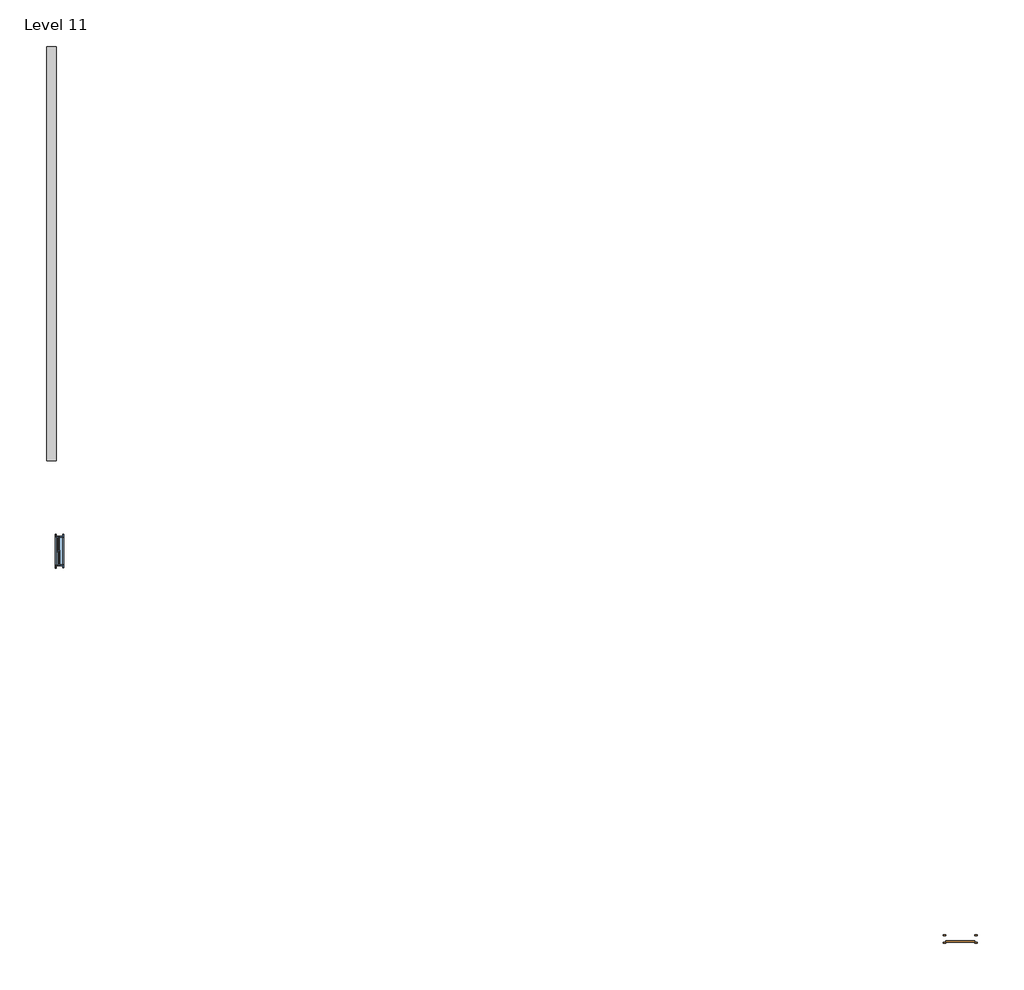
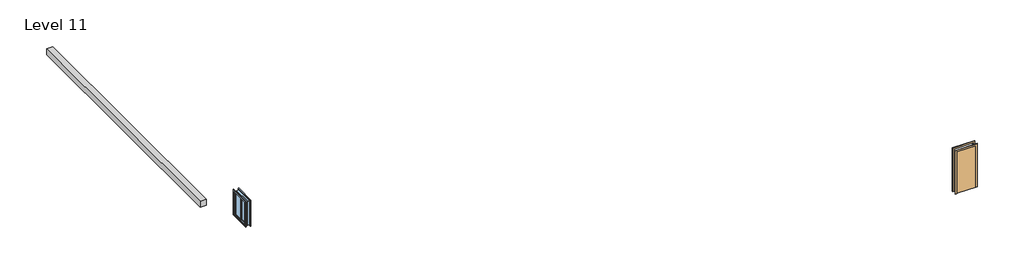
# One storey: 1 door, 1 proxy, 1 window.
"""IFC4 building model written with IfcOpenShell, lengths in millimetres."""

from ifc_helpers import new_model, si_unit, origin, place, context, project, spatial, transform, mapped, element, save
from components import generic_models_18_generic_models_18_cf5f2b29, door_719f80de, window_54100e87

model = new_model("IFC4")

# Units and contexts
model_context = context("Model", 3, world=origin())
ifc_project = project(units=[si_unit("LENGTHUNIT", "METRE", prefix="MILLI")], contexts=[model_context])

# Site, building, storey
site = spatial("IfcSite", under=ifc_project)
building = spatial("IfcBuilding", under=site)
storey = spatial("IfcBuildingStorey", under=building, Name="Level 11", Elevation=19507.2)

# Proxy
placement = place(None, origin())
generic_models_18_generic_models_18_shape = generic_models_18_generic_models_18_cf5f2b29(model_context)
element("IfcBuildingElementProxy", 1, Name="Generic Models 18 : Generic Models 18", ObjectType="Generic Models 18 : Generic Models 18", at=placement, inside=storey, context=model_context, shape_type="MappedRepresentation", body=[
    mapped(generic_models_18_generic_models_18_shape, transform((0.0, 0.0, 0.0), x_axis=(1.0, 0.0, 0.0), y_axis=(0.0, 1.0, 0.0), z_axis=(0.0, 0.0, 1.0))),
])

# Door
door_shape = door_719f80de(model_context)
element("IfcDoor", 2, ObjectType="Single-Flush : 36\" x 84\"", at=placement, inside=storey, context=model_context, shape_type="MappedRepresentation", body=[
    mapped(door_shape, transform((12764.961926, -20744.1985361, 19507.2), x_axis=(1.0, 0.0, 0.0), y_axis=(0.0, 1.0, 0.0), z_axis=(0.0, 0.0, 1.0))),
])

# Window
window_shape = window_54100e87(model_context)
element("IfcWindow", 3, ObjectType="Slider with Trim : 36\" x 48\"", at=placement, inside=storey, context=model_context, shape_type="MappedRepresentation", body=[
    mapped(window_shape, transform((-15175.038074, -8710.0213044, 19507.2), x_axis=(0.0, 1.0, 0.0), y_axis=(-1.0, 0.0, 0.0), z_axis=(0.0, 0.0, 1.0))),
])

save(model, "model.ifc")

# Revit data of these elements
# Type "Single-Flush : 36\" x 84\""
#   Type Mark = "1"
#   Construction Type Id = "MDOOR"
#   Assembly Code = "C1020"
#   Analytic Construction = "Metal"
#   Thickness = 0' - 2"
#   Heat Transfer Coefficient (U) = 0.651978 BTU/(h·ft²·°F)
#   Height = 7' - 0"
#   Trim Projection Ext = 0' - 1"
#   Trim Projection Int = 0' - 1"
#   Trim Width = 0' - 3"
#   Width = 3' - 0"
#   Define Thermal Properties by = 1
#   Door Material = Door - Panel
#   Frame Material = Door - Frame
#   Visual Light Transmittance = 0
#   Solar Heat Gain Coefficient = 0
#   Function = (empty or 0)
#   Wall Closure = (empty or 0)
# Type "Slider with Trim : 36\" x 48\""
#   Type Mark = "22"
#   Construction Type Id = "GSP4R"
#   Assembly Code = "B2020100"
#   Analytic Construction = "1/8 in Pilkington single glazing"
#   Visual Light Transmittance = 0.9
#   Solar Heat Gain Coefficient = 0.78
#   Heat Transfer Coefficient (U) = 0.6496 BTU/(h·ft²·°F)
#   Height = 4' - 0"
#   Default Sill Height = 3' - 0"
#   Trim Projection - Ext. = 0' - 0 3/4"
#   Trim Projection - Int. = 0' - 0 3/4"
#   Trim Width - Exterior = 0' - 3 1/2"
#   Trim Width - Interior = 0' - 3 1/2"
#   Width = 3' - 0"
#   Window Inset = 0' - 0 3/4"
#   Define Thermal Properties by = 1
#   Glass Pane Material = Glass
#   Sash Material = Sash
#   Trim Exterior Material = Trim
#   Trim Interior Material = Trim
#   Wall Closure = (empty or 0)
# Element 1 (IfcBuildingElementProxy, "Generic Models 18 : Generic Models 18")
#   Phase Created = New Construction
# Element 2 (IfcDoor, "Single-Flush : 36\" x 84\"")
#   Phase Created = New Construction
#   Materials on its faces: "Door - Frame", "Door - Panel"
# Element 3 (IfcWindow, "Slider with Trim : 36\" x 48\"")
#   Mark = "39"
#   Phase Created = New Construction
#   Materials on its faces: "Sash", "Trim", "Glass"
# Materials
#   "Door - Panel": class "Wood", colour RGB 210 159 95, transparency 0
#   "Door - Frame": colour RGB 118 70 51, transparency 0
#   "Glass": class "Glass", colour RGB 0 128 192, transparency 0.75, Description = "Soda Lime Glass", Cost = 0
#   "Sash": class "Wood", colour RGB 224 178 126, transparency 0
#   "Trim": class "Wood", colour RGB 224 178 126, transparency 0
